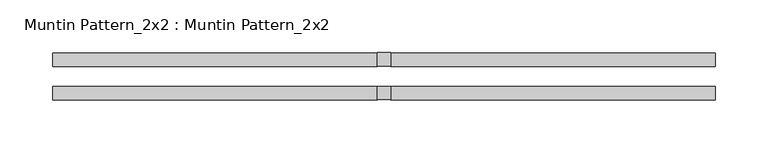
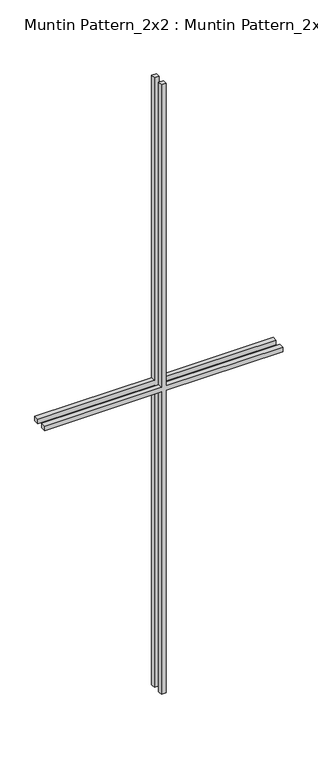
"""IFC4 building model written with IfcOpenShell, lengths in millimetres: proxy geometry, Muntin Pattern_2x2 : Muntin Pattern_2x2."""

from ifc_helpers import new_model, si_unit, frame, origin, place, context, project, spatial, polyline, outline, extrude, source, transform, mapped, element, save


def muntin_pattern_2x2_muntin_pattern_2x2_f6a80940(model_context):
    return source(origin(), model_context, "Body", "SweptSolid", [
        extrude(outline(polyline([(850.9, -6.35), (850.9, -312.7375), (838.2, -312.7375), (838.2, -6.35), (0.0, -6.35), (0.0, 6.35), (838.2, 6.35), (838.2, 312.7375), (850.9, 312.7375), (850.9, 6.35), (1689.1, 6.35), (1689.1, -6.35), (850.9, -6.35)])), frame((0.0, 9.525, 0.0), z_axis=(0.0, 1.0, 0.0), x_axis=(0.0, 0.0, 1.0)), (0.0, 0.0, 1.0), 12.7),
        extrude(outline(polyline([(850.9, -6.35), (850.9, -312.7375), (838.2, -312.7375), (838.2, -6.35), (0.0, -6.35), (0.0, 6.35), (838.2, 6.35), (838.2, 312.7375), (850.9, 312.7375), (850.9, 6.35), (1689.1, 6.35), (1689.1, -6.35), (850.9, -6.35)])), frame((0.0, -22.225, 0.0), z_axis=(0.0, 1.0, 0.0), x_axis=(0.0, 0.0, 1.0)), (0.0, 0.0, 1.0), 12.7),
    ])


if __name__ == "__main__":
    model = new_model("IFC4")
    model_context = context("Model", 3, world=origin())
    ifc_project = project(units=[si_unit("LENGTHUNIT", "METRE", prefix="MILLI")], contexts=[model_context])
    site = spatial("IfcSite", under=ifc_project)
    building = spatial("IfcBuilding", under=site)
    placement = place(None, origin())
    muntin_pattern_2x2_muntin_pattern_2x2_shape = muntin_pattern_2x2_muntin_pattern_2x2_f6a80940(model_context)
    element("IfcBuildingElementProxy", 1, Name="Muntin Pattern_2x2 : Muntin Pattern_2x2", ObjectType="Muntin Pattern_2x2 : Muntin Pattern_2x2", at=placement, inside=building, context=model_context, shape_type="MappedRepresentation", body=[
        mapped(muntin_pattern_2x2_muntin_pattern_2x2_shape, transform((0.0, 0.0, 0.0), x_axis=(1.0, 0.0, 0.0), y_axis=(0.0, 1.0, 0.0), z_axis=(0.0, 0.0, 1.0))),
    ])
    save(model, "model.ifc")

# Revit data of these elements
# Type "Muntin Pattern_2x2 : Muntin Pattern_2x2"
#   Width [instance default] = 4' - 0"
#   Thickness = 0' - 0 1/2"
#   Height [instance default] = 4' - 0"
#   Distance = 0' - 0 3/4"
#   Interior Material [instance default] = none
#   Exterior Material [instance default] = none
#   Default Elevation = 0
# Element 1 (IfcBuildingElementProxy, "Muntin Pattern_2x2 : Muntin Pattern_2x2")
#   Width = 2' - 0 5/8"
#   Height = 5' - 6 1/2"
#   Interior Material = Wood - Stained
#   Exterior Material = Clad - White
#   Materials on its faces: "Clad - White", "Wood - Stained"
# Materials
#   "Clad - White": class "Wood", colour RGB 242 242 238, transparency 0, Cost = 0
#   "Wood - Stained": class "Wood", colour RGB 224 178 126, transparency 0, Cost = 0
